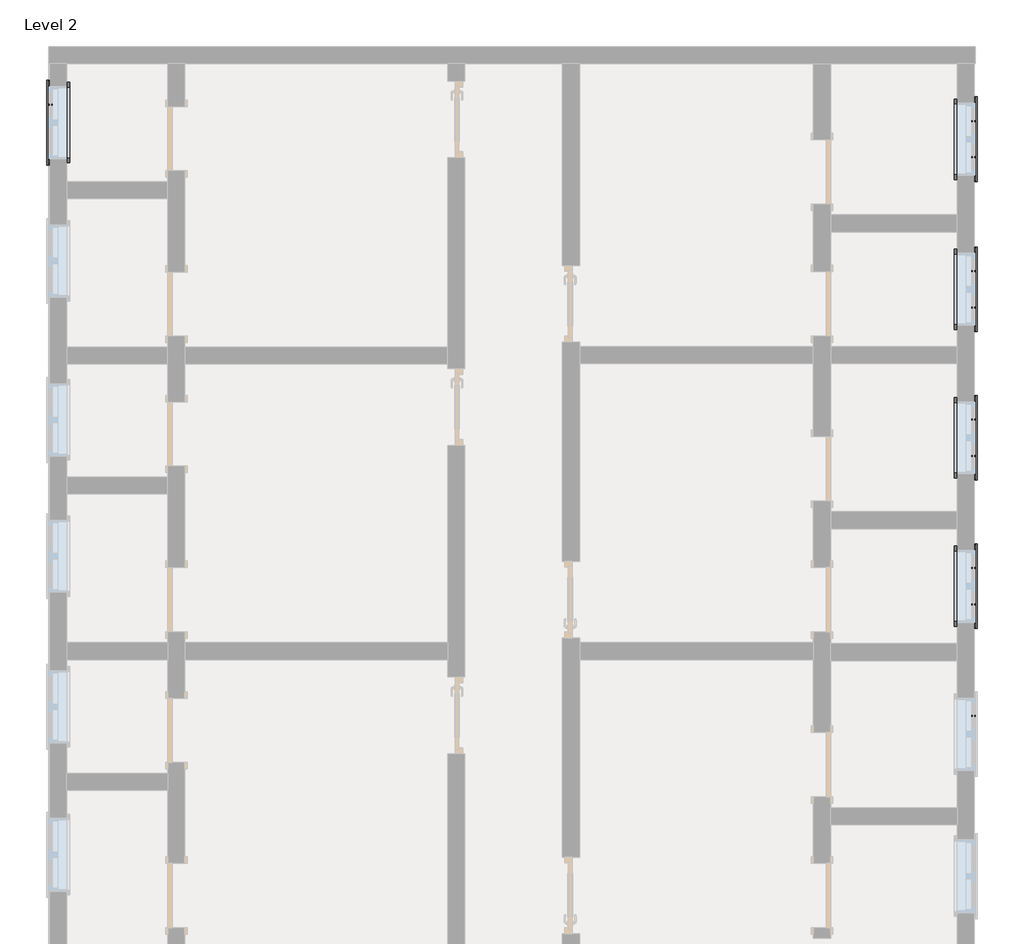
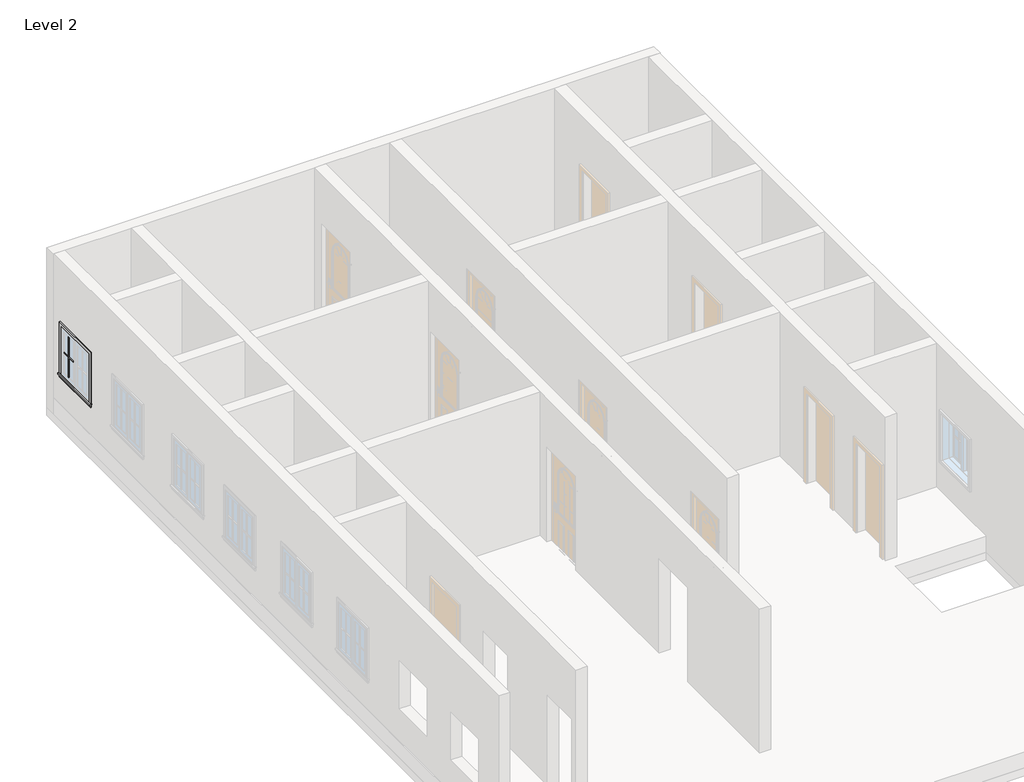
# One storey, part 4 of 4: 20 proxies.
"""IFC4 building model written with IfcOpenShell, lengths in millimetres."""

from ifc_helpers import new_model, si_unit, origin, place, context, project, spatial, transform, mapped, element, save
from components import muntin_pattern_2x2_muntin_pattern_2x2_b3fe6957, muntin_pattern_2x2_muntin_pattern_2x2_3e0ecaf2, trim_window_exterior_flat_with_sill_41619996, trim_window_interior_flat_picture_frame_51c85655

model = new_model("IFC4")

# Units and contexts
model_context = context("Model", 3, world=origin())
ifc_project = project(units=[si_unit("LENGTHUNIT", "METRE", prefix="MILLI")], contexts=[model_context])

# Site, building, storey
site = spatial("IfcSite", under=ifc_project)
building = spatial("IfcBuilding", under=site)
storey = spatial("IfcBuildingStorey", under=building, Name="Level 2", Elevation=3048.0)

# Proxies
placement = place(None, origin())
muntin_pattern_2x2_muntin_pattern_2x2_shape = muntin_pattern_2x2_muntin_pattern_2x2_b3fe6957(model_context)
element("IfcBuildingElementProxy", 1, Name="Muntin Pattern_2x2 : Muntin Pattern_2x2", ObjectType="Muntin Pattern_2x2 : Muntin Pattern_2x2", at=placement, inside=storey, context=model_context, shape_type="MappedRepresentation", body=[
    mapped(muntin_pattern_2x2_muntin_pattern_2x2_shape, transform((4489.4641134, 66.1024728, 4032.25), x_axis=(0.0, -1.0, 0.0), y_axis=(1.0, 0.0, 0.0), z_axis=(0.0, 0.0, 1.0))),
])
element("IfcBuildingElementProxy", 2, Name="Muntin Pattern_2x2 : Muntin Pattern_2x2", ObjectType="Muntin Pattern_2x2 : Muntin Pattern_2x2", at=placement, inside=storey, context=model_context, shape_type="MappedRepresentation", body=[
    mapped(muntin_pattern_2x2_muntin_pattern_2x2_shape, transform((4489.4641134, 1818.7024728, 4032.25), x_axis=(0.0, -1.0, 0.0), y_axis=(1.0, 0.0, 0.0), z_axis=(0.0, 0.0, 1.0))),
])
element("IfcBuildingElementProxy", 3, Name="Muntin Pattern_2x2 : Muntin Pattern_2x2", ObjectType="Muntin Pattern_2x2 : Muntin Pattern_2x2", at=placement, inside=storey, context=model_context, shape_type="MappedRepresentation", body=[
    mapped(muntin_pattern_2x2_muntin_pattern_2x2_shape, transform((4489.4641134, 3577.6524728, 4032.25), x_axis=(0.0, -1.0, 0.0), y_axis=(1.0, 0.0, 0.0), z_axis=(0.0, 0.0, 1.0))),
])
element("IfcBuildingElementProxy", 4, Name="Muntin Pattern_2x2 : Muntin Pattern_2x2", ObjectType="Muntin Pattern_2x2 : Muntin Pattern_2x2", at=placement, inside=storey, context=model_context, shape_type="MappedRepresentation", body=[
    mapped(muntin_pattern_2x2_muntin_pattern_2x2_shape, transform((4489.4641134, 5336.6024728, 4032.25), x_axis=(0.0, -1.0, 0.0), y_axis=(1.0, 0.0, 0.0), z_axis=(0.0, 0.0, 1.0))),
])
element("IfcBuildingElementProxy", 5, Name="Muntin Pattern_2x2 : Muntin Pattern_2x2", ObjectType="Muntin Pattern_2x2 : Muntin Pattern_2x2", at=placement, inside=storey, context=model_context, shape_type="MappedRepresentation", body=[
    mapped(muntin_pattern_2x2_muntin_pattern_2x2_shape, transform((4489.4641134, 7114.6024728, 4032.25), x_axis=(0.0, -1.0, 0.0), y_axis=(1.0, 0.0, 0.0), z_axis=(0.0, 0.0, 1.0))),
])
muntin_pattern_2x2_muntin_pattern_2x2_2_shape = muntin_pattern_2x2_muntin_pattern_2x2_3e0ecaf2(model_context)
element("IfcBuildingElementProxy", 6, Name="Muntin Pattern_2x2 : Muntin Pattern_2x2", ObjectType="Muntin Pattern_2x2 : Muntin Pattern_2x2", at=placement, inside=storey, context=model_context, shape_type="MappedRepresentation", body=[
    mapped(muntin_pattern_2x2_muntin_pattern_2x2_2_shape, transform((-6438.8858866, 7311.4524728, 4032.25), x_axis=(0.0, -1.0, 0.0), y_axis=(1.0, 0.0, 0.0), z_axis=(0.0, 0.0, 1.0))),
])
element("IfcBuildingElementProxy", 7, Name="Muntin Pattern_2x2 : Muntin Pattern_2x2", ObjectType="Muntin Pattern_2x2 : Muntin Pattern_2x2", at=placement, inside=storey, context=model_context, shape_type="MappedRepresentation", body=[
    mapped(muntin_pattern_2x2_muntin_pattern_2x2_2_shape, transform((4489.4641134, 1390.0774728, 4032.25), x_axis=(0.0, 1.0, 0.0), y_axis=(-1.0, 0.0, 0.0), z_axis=(0.0, 0.0, 1.0))),
])
element("IfcBuildingElementProxy", 8, Name="Muntin Pattern_2x2 : Muntin Pattern_2x2", ObjectType="Muntin Pattern_2x2 : Muntin Pattern_2x2", at=placement, inside=storey, context=model_context, shape_type="MappedRepresentation", body=[
    mapped(muntin_pattern_2x2_muntin_pattern_2x2_2_shape, transform((4489.4641134, 3149.0274728, 4032.25), x_axis=(0.0, 1.0, 0.0), y_axis=(-1.0, 0.0, 0.0), z_axis=(0.0, 0.0, 1.0))),
])
element("IfcBuildingElementProxy", 9, Name="Muntin Pattern_2x2 : Muntin Pattern_2x2", ObjectType="Muntin Pattern_2x2 : Muntin Pattern_2x2", at=placement, inside=storey, context=model_context, shape_type="MappedRepresentation", body=[
    mapped(muntin_pattern_2x2_muntin_pattern_2x2_2_shape, transform((4489.4641134, 4907.9774728, 4032.25), x_axis=(0.0, 1.0, 0.0), y_axis=(-1.0, 0.0, 0.0), z_axis=(0.0, 0.0, 1.0))),
])
element("IfcBuildingElementProxy", 10, Name="Muntin Pattern_2x2 : Muntin Pattern_2x2", ObjectType="Muntin Pattern_2x2 : Muntin Pattern_2x2", at=placement, inside=storey, context=model_context, shape_type="MappedRepresentation", body=[
    mapped(muntin_pattern_2x2_muntin_pattern_2x2_2_shape, transform((4489.4641134, 6685.9774728, 4032.25), x_axis=(0.0, 1.0, 0.0), y_axis=(-1.0, 0.0, 0.0), z_axis=(0.0, 0.0, 1.0))),
])
trim_window_exterior_flat_with_sill_shape = trim_window_exterior_flat_with_sill_41619996(model_context)
element("IfcBuildingElementProxy", 11, Name="Trim-Window-Exterior-Flat : with Sill", ObjectType="Trim-Window-Exterior-Flat : with Sill", at=placement, inside=storey, context=model_context, shape_type="MappedRepresentation", body=[
    mapped(trim_window_exterior_flat_with_sill_shape, transform((-6448.4108866, 7097.1399728, 4876.8), x_axis=(0.0, -1.0, 0.0), y_axis=(0.0, 0.0, 1.0), z_axis=(-1.0, 0.0, 0.0))),
])
element("IfcBuildingElementProxy", 12, Name="Trim-Window-Exterior-Flat : with Sill", ObjectType="Trim-Window-Exterior-Flat : with Sill", at=placement, inside=storey, context=model_context, shape_type="MappedRepresentation", body=[
    mapped(trim_window_exterior_flat_with_sill_shape, transform((4498.9891134, 1604.3899728, 4876.8), x_axis=(0.0, 1.0, 0.0), y_axis=(0.0, 0.0, 1.0), z_axis=(1.0, 0.0, 0.0))),
])
element("IfcBuildingElementProxy", 13, Name="Trim-Window-Exterior-Flat : with Sill", ObjectType="Trim-Window-Exterior-Flat : with Sill", at=placement, inside=storey, context=model_context, shape_type="MappedRepresentation", body=[
    mapped(trim_window_exterior_flat_with_sill_shape, transform((4498.9891134, 3363.3399728, 4876.8), x_axis=(0.0, 1.0, 0.0), y_axis=(0.0, 0.0, 1.0), z_axis=(1.0, 0.0, 0.0))),
])
element("IfcBuildingElementProxy", 14, Name="Trim-Window-Exterior-Flat : with Sill", ObjectType="Trim-Window-Exterior-Flat : with Sill", at=placement, inside=storey, context=model_context, shape_type="MappedRepresentation", body=[
    mapped(trim_window_exterior_flat_with_sill_shape, transform((4498.9891134, 5122.2899728, 4876.8), x_axis=(0.0, 1.0, 0.0), y_axis=(0.0, 0.0, 1.0), z_axis=(1.0, 0.0, 0.0))),
])
element("IfcBuildingElementProxy", 15, Name="Trim-Window-Exterior-Flat : with Sill", ObjectType="Trim-Window-Exterior-Flat : with Sill", at=placement, inside=storey, context=model_context, shape_type="MappedRepresentation", body=[
    mapped(trim_window_exterior_flat_with_sill_shape, transform((4498.9891134, 6900.2899728, 4876.8), x_axis=(0.0, 1.0, 0.0), y_axis=(0.0, 0.0, 1.0), z_axis=(1.0, 0.0, 0.0))),
])
trim_window_interior_flat_picture_frame_shape = trim_window_interior_flat_picture_frame_51c85655(model_context)
element("IfcBuildingElementProxy", 16, Name="Trim-Window-Interior-Flat : Picture Frame", ObjectType="Trim-Window-Interior-Flat : Picture Frame", at=placement, inside=storey, context=model_context, shape_type="MappedRepresentation", body=[
    mapped(trim_window_interior_flat_picture_frame_shape, transform((-6245.2108866, 7097.1399728, 4876.8), x_axis=(0.0, 1.0, 0.0), y_axis=(0.0, 0.0, 1.0), z_axis=(1.0, 0.0, 0.0))),
])
element("IfcBuildingElementProxy", 17, Name="Trim-Window-Interior-Flat : Picture Frame", ObjectType="Trim-Window-Interior-Flat : Picture Frame", at=placement, inside=storey, context=model_context, shape_type="MappedRepresentation", body=[
    mapped(trim_window_interior_flat_picture_frame_shape, transform((4295.7891134, 1604.3899728, 4876.8), x_axis=(0.0, -1.0, 0.0), y_axis=(0.0, 0.0, 1.0), z_axis=(-1.0, 0.0, 0.0))),
])
element("IfcBuildingElementProxy", 18, Name="Trim-Window-Interior-Flat : Picture Frame", ObjectType="Trim-Window-Interior-Flat : Picture Frame", at=placement, inside=storey, context=model_context, shape_type="MappedRepresentation", body=[
    mapped(trim_window_interior_flat_picture_frame_shape, transform((4295.7891134, 3363.3399728, 4876.8), x_axis=(0.0, -1.0, 0.0), y_axis=(0.0, 0.0, 1.0), z_axis=(-1.0, 0.0, 0.0))),
])
element("IfcBuildingElementProxy", 19, Name="Trim-Window-Interior-Flat : Picture Frame", ObjectType="Trim-Window-Interior-Flat : Picture Frame", at=placement, inside=storey, context=model_context, shape_type="MappedRepresentation", body=[
    mapped(trim_window_interior_flat_picture_frame_shape, transform((4295.7891134, 5122.2899728, 4876.8), x_axis=(0.0, -1.0, 0.0), y_axis=(0.0, 0.0, 1.0), z_axis=(-1.0, 0.0, 0.0))),
])
element("IfcBuildingElementProxy", 20, Name="Trim-Window-Interior-Flat : Picture Frame", ObjectType="Trim-Window-Interior-Flat : Picture Frame", at=placement, inside=storey, context=model_context, shape_type="MappedRepresentation", body=[
    mapped(trim_window_interior_flat_picture_frame_shape, transform((4295.7891134, 6900.2899728, 4876.8), x_axis=(0.0, -1.0, 0.0), y_axis=(0.0, 0.0, 1.0), z_axis=(-1.0, 0.0, 0.0))),
])

save(model, "model.ifc")

# Revit data of these elements
# Type "Muntin Pattern_2x2 : Muntin Pattern_2x2"
#   Width [instance default] = 4' - 0"
#   Thickness = 0' - 0 1/2"
#   Height [instance default] = 4' - 0"
#   Distance = 0' - 0 3/4"
#   Interior Material [instance default] = none
#   Exterior Material [instance default] = none
#   Default Elevation = 0
# Type "Trim-Window-Exterior-Flat : with Sill"
#   Trim Width = 0' - 2 1/4"
#   Trim Thickness_Picture Frame = 0' - 1 1/4"
#   Trim Thickness_with Sill = 0' - 0 3/4"
#   Sill Thickness = 0' - 1 1/4"
#   Opening Width [instance default] = 2' - 0"
#   Opening Height [instance default] = 3' - 0"
#   Default Elevation = 4' - 0"
#   Sill = yes
#   Picture Frame = no
#   Trim Material [instance default] = none
# Type "Trim-Window-Interior-Flat : Picture Frame"
#   Trim Thickness_Picture Frame = 0' - 1 1/4"
#   Trim Width = 0' - 2 1/4"
#   Trim Thickness_with Sill = 0' - 0 3/4"
#   Sill Thickness = 0' - 1 1/4"
#   Opening Width [instance default] = 2' - 0"
#   Opening Height [instance default] = 3' - 0"
#   Default Elevation = 4' - 0"
#   Sill = no
#   Picture Frame = yes
#   Trim Material [instance default] = none
# Elements 1, 2, 3, 4, 5, 6, 7, 8, 9, 10 (IfcBuildingElementProxy, "Muntin Pattern_2x2 : Muntin Pattern_2x2")
#   Width = 0' - 11 5/8"
#   Height = 2' - 6 1/2"
#   Interior Material = Wood - Stained
#   Exterior Material = Clad - White
#   Phase Created = New Construction
#   Materials on its faces: "Clad - White", "Wood - Stained"
# Elements 11, 12, 13, 14, 15 (IfcBuildingElementProxy, "Trim-Window-Exterior-Flat : with Sill")
#   Opening Width = 2' - 10"
#   Opening Height = 3' - 0"
#   Trim Material = Clad - White
#   Phase Created = New Construction
#   Materials on its faces: "Clad - White"
# Elements 16, 17, 18, 19, 20 (IfcBuildingElementProxy, "Trim-Window-Interior-Flat : Picture Frame")
#   Opening Width = 2' - 10"
#   Opening Height = 3' - 0"
#   Trim Material = Wood - Stained
#   Phase Created = New Construction
#   Materials on its faces: "Wood - Stained"
# Materials
#   "Clad - White": class "Wood", colour RGB 242 242 238, transparency 0, Cost = 0
#   "Wood - Stained": class "Wood", colour RGB 224 178 126, transparency 0, Cost = 0
